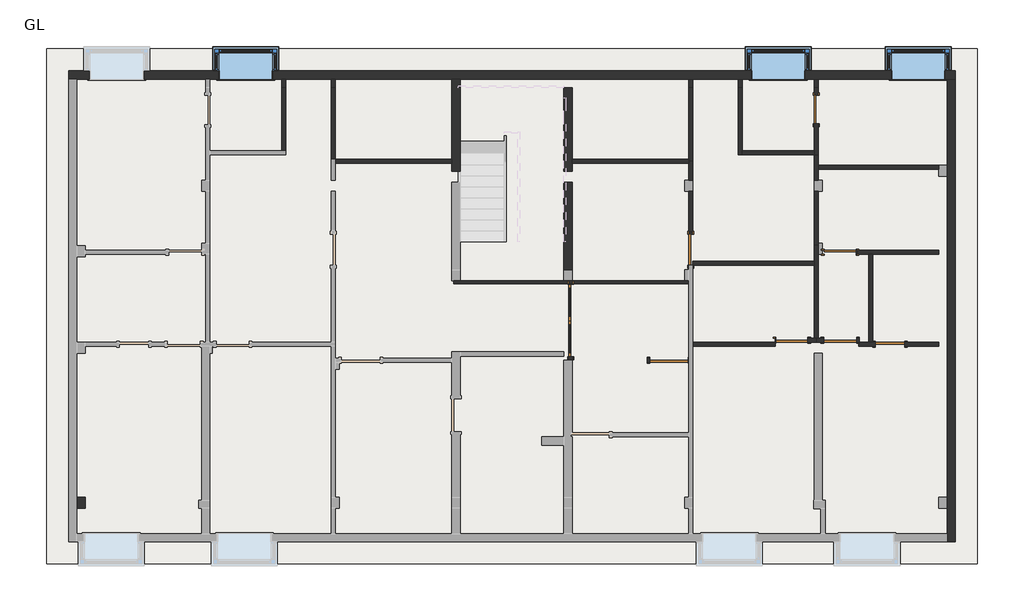
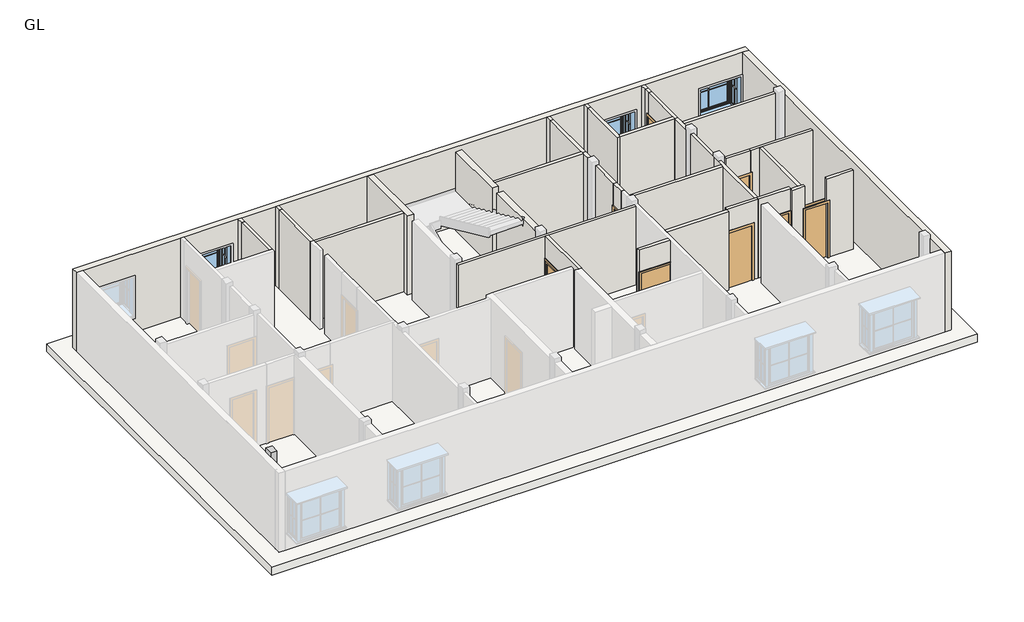
# One storey, part 2 of 3: 38 walls, 8 doors, 3 windows, 1 column, 1 slab.
"""IFC4 building model written with IfcOpenShell, lengths in millimetres."""

from ifc_helpers import new_model, si_unit, frame, origin, place, context, project, spatial, polyline, outline, extrude, faceted_brep, transform, mapped, element, save
from components import door_04ab2522, m_door_single_panel_05506f71, door_85b31ab1, door_1991e9a2, door_a431d384, door_82def9da, m_door_single_panel_3_x7_f8176753, window_19bbd869

model = new_model("IFC4")

# Units and contexts
model_context = context("Model", 3, world=origin())
ifc_project = project(units=[si_unit("LENGTHUNIT", "METRE", prefix="MILLI")], contexts=[model_context])

# Site, building, storey
site = spatial("IfcSite", under=ifc_project)
building = spatial("IfcBuilding", under=site)
storey = spatial("IfcBuildingStorey", under=building, Name="GL", Elevation=3200.4)

# Column
placement = place(None, origin())
element("IfcColumn", 1, ObjectType="Rectangular Column : 1'X 9\"", at=placement, inside=storey, context=model_context, shape_type="SweptSolid", body=[
    extrude(outline(polyline([(-12224.6987957, -3709.2932671), (-12224.6987957, -4014.0932671), (-12453.2987957, -4014.0932671), (-12453.2987957, -3709.2932671), (-12224.6987957, -3709.2932671)])), frame((0.0, 0.0, 3200.4), z_axis=(0.0, 0.0, 1.0), x_axis=(1.0, 0.0, 0.0)), (0.0, 0.0, 1.0), 3200.4),
])

# Doors
door_shape = door_04ab2522(model_context)
element("IfcDoor", 2, ObjectType="M_Door-Double-Glass : 6'7\"X7'", at=placement, inside=storey, context=model_context, shape_type="MappedRepresentation", body=[
    mapped(door_shape, transform((1217.5394962, 1183.3817656, 3200.4), x_axis=(0.0, 1.0, 0.0), y_axis=(-1.0, 0.0, 0.0), z_axis=(0.0, 0.0, 1.0))),
])
m_door_single_panel_shape = m_door_single_panel_05506f71(model_context)
element("IfcDoor", 3, ObjectType="M_Door-Single-Panel", at=placement, inside=storey, context=model_context, shape_type="MappedRepresentation", body=[
    mapped(m_door_single_panel_shape, transform((3933.4813133, 90.9578621, 3200.4), x_axis=(1.0, 0.0, 0.0), y_axis=(0.0, 1.0, 0.0), z_axis=(0.0, 0.0, 1.0))),
])
door_2_shape = door_85b31ab1(model_context)
element("IfcDoor", 4, ObjectType="M_Door-Single-Panel : 2'10\"X7' 2", at=placement, inside=storey, context=model_context, shape_type="MappedRepresentation", body=[
    mapped(door_2_shape, transform((4532.9512082, 3142.9626891, 3200.4), x_axis=(0.0, -1.0, 0.0), y_axis=(1.0, 0.0, 0.0), z_axis=(0.0, 0.0, 1.0))),
])
door_3_shape = door_1991e9a2(model_context)
element("IfcDoor", 5, ObjectType="M_Door-Single-Panel : 2'11\"X7' 3", at=placement, inside=storey, context=model_context, shape_type="MappedRepresentation", body=[
    mapped(door_3_shape, transform((7330.1405552, 640.4567334, 3200.4), x_axis=(1.0, 0.0, 0.0), y_axis=(0.0, 1.0, 0.0), z_axis=(0.0, 0.0, 1.0))),
])
element("IfcDoor", 6, ObjectType="M_Door-Single-Panel : 2'11\"X7' 3", at=placement, inside=storey, context=model_context, shape_type="MappedRepresentation", body=[
    mapped(door_3_shape, transform((8664.274939, 3078.8567332, 3200.4), x_axis=(-1.0, 0.0, 0.0), y_axis=(0.0, -1.0, 0.0), z_axis=(0.0, 0.0, 1.0))),
])
door_4_shape = door_a431d384(model_context)
element("IfcDoor", 7, ObjectType="M_Door-Single-Panel : 2'7\"X7' 2", at=placement, inside=storey, context=model_context, shape_type="MappedRepresentation", body=[
    mapped(door_4_shape, transform((8000.0512079, 7021.3751452, 3200.4), x_axis=(0.0, 1.0, 0.0), y_axis=(-1.0, 0.0, 0.0), z_axis=(0.0, 0.0, 1.0))),
])
door_5_shape = door_82def9da(model_context)
element("IfcDoor", 8, ObjectType="M_Door-Single-Panel : 2'8\"X7'", at=placement, inside=storey, context=model_context, shape_type="MappedRepresentation", body=[
    mapped(door_5_shape, transform((10046.0486694, 526.1567295, 3200.4), x_axis=(-1.0, 0.0, 0.0), y_axis=(0.0, -1.0, 0.0), z_axis=(0.0, 0.0, 1.0))),
])
m_door_single_panel_3_x7_shape = m_door_single_panel_3_x7_f8176753(model_context)
element("IfcDoor", 9, ObjectType="M_Door-Single-Panel : 3'X7'", at=placement, inside=storey, context=model_context, shape_type="MappedRepresentation", body=[
    mapped(m_door_single_panel_3_x7_shape, transform((8666.8012079, 640.4567334, 3200.4), x_axis=(-1.0, 0.0, 0.0), y_axis=(0.0, -1.0, 0.0), z_axis=(0.0, 0.0, 1.0))),
])

# Slab
element("IfcSlab", 10, ObjectType="Generic - 12\"", at=placement, inside=storey, context=model_context, shape_type="SweptSolid", body=[
    extrude(outline(polyline([(12464.1012075, 8698.6067329), (12464.1012075, -5550.7932662), (-13291.4987957, -5550.7932662), (-13291.4987957, 8698.6067329), (12464.1012075, 8698.6067329)])), frame((0.0, 0.0, 2895.6), z_axis=(0.0, 0.0, 1.0), x_axis=(1.0, 0.0, 0.0)), (0.0, 0.0, 1.0), 304.8),
])

# Walls
element("IfcWall", 11, ObjectType="3.5\"", at=placement, inside=storey, context=model_context, shape_type="Brep", body=[
    faceted_brep([(-2020.2487998, 2196.2067742, 3200.4), (1158.0082462, 2196.2067742, 3200.4), (1272.3082462, 2196.2067742, 3200.4), (4475.8012082, 2196.2067742, 3200.4), (4475.8012082, 2196.2067742, 6248.4), (1272.3082462, 2196.2067742, 6248.4), (1158.0082462, 2196.2067742, 6248.4), (-2020.2487998, 2196.2067742, 6248.4), (-2020.2487998, 2285.1067742, 3200.4), (-2020.2487998, 2285.1067742, 6248.4), (4475.8012082, 2285.1067742, 6248.4), (4475.8012082, 2285.1067742, 3200.4), (4361.5012082, 2285.1067742, 3200.4), (1253.2582462, 2285.1067742, 3200.4), (1024.6582462, 2285.1067742, 3200.4), (-1845.5417538, 2285.1067742, 3200.4)], [[[0, 1, 2, 3, 4, 5, 6, 7]], [[8, 9, 10, 11, 12, 13, 14, 15]], [[3, 2, 1, 0, 8, 15, 14, 13, 12, 11]], [[7, 6, 5, 4, 10, 9]], [[0, 7, 9, 8]], [[4, 3, 11, 10]]]),
])
element("IfcWall", 12, ObjectType="4.5\"", at=placement, inside=storey, context=model_context, shape_type="SweptSolid", body=[
    extrude(outline(polyline([(3132.0737955, 6248.4), (3628.3344162, 6248.4), (3628.3344162, 3200.4), (3574.7626891, 3200.4), (3574.7626891, 5334.0), (3132.0737955, 5334.0), (3132.0737955, 6248.4)])), frame((4475.8012082, 0.0, 0.0), z_axis=(1.0, 0.0, 0.0), x_axis=(0.0, 1.0, 0.0)), (0.0, 0.0, 1.0), 114.3),
])
element("IfcWall", 13, ObjectType="4.5\"", at=placement, inside=storey, context=model_context, shape_type="Brep", body=[
    faceted_brep([(8000.0512079, 583.3067334, 3200.4), (8000.0512079, 583.3067334, 6248.4), (6862.7668241, 583.3067334, 6248.4), (6862.7668241, 583.3067334, 3200.4), (6885.6405552, 583.3067334, 3200.4), (6885.6405552, 583.3067334, 5334.0), (7774.6405552, 583.3067334, 5334.0), (7774.6405552, 583.3067334, 3200.4), (8000.0512079, 697.6067334, 6248.4), (8000.0512079, 697.6067334, 3200.4), (7942.9012079, 697.6067334, 3200.4), (7774.6405552, 697.6067334, 3200.4), (7774.6405552, 697.6067334, 5334.0), (6885.6405552, 697.6067334, 5334.0), (6885.6405552, 697.6067334, 3200.4), (6862.7668241, 697.6067334, 3200.4), (6862.7668241, 697.6067334, 6248.4), (7942.9012079, 697.6067334, 6248.4)], [[[0, 1, 2, 3, 4, 5, 6, 7]], [[8, 9, 10, 11, 12, 13, 14, 15, 16, 17]], [[3, 15, 14, 4]], [[9, 0, 7, 11, 10]], [[1, 0, 9, 8]], [[2, 1, 8, 17, 16]], [[3, 2, 16, 15]], [[6, 12, 11, 7]], [[12, 6, 5, 13]], [[13, 5, 4, 14]]]),
])
element("IfcWall", 14, ObjectType="4.5\"", at=placement, inside=storey, context=model_context, shape_type="Brep", body=[
    faceted_brep([(9187.5012047, 583.3067334, 3200.4), (9187.5012047, 583.3067334, 6248.4), (8000.0512079, 583.3067334, 6248.4), (8000.0512079, 583.3067334, 3200.4), (8209.6012079, 583.3067334, 3200.4), (8209.6012079, 583.3067334, 5334.0), (9124.0012079, 583.3067334, 5334.0), (9124.0012079, 583.3067334, 3200.4), (9187.5012047, 697.6067334, 6248.4), (9187.5012047, 697.6067334, 3200.4), (9124.0012079, 697.6067334, 3200.4), (9124.0012079, 697.6067334, 5334.0), (8209.6012079, 697.6067334, 5334.0), (8209.6012079, 697.6067334, 3200.4), (8057.2012079, 697.6067334, 3200.4), (8000.0512079, 697.6067334, 3200.4), (8000.0512079, 697.6067334, 6248.4), (8057.2012079, 697.6067334, 6248.4)], [[[0, 1, 2, 3, 4, 5, 6, 7]], [[8, 9, 10, 11, 12, 13, 14, 15, 16, 17]], [[9, 0, 7, 10]], [[3, 15, 14, 13, 4]], [[1, 0, 9, 8]], [[2, 1, 8, 17, 16]], [[3, 2, 16, 15]], [[5, 12, 11, 6]], [[6, 11, 10, 7]], [[12, 5, 4, 13]]]),
])
element("IfcWall", 15, ObjectType="4.5\"", at=placement, inside=storey, context=model_context, shape_type="SweptSolid", body=[
    extrude(outline(polyline([(3200.4, 9131.6486701), (6248.4, 9131.6486701), (6248.4, 8245.174939), (5334.0, 8245.174939), (5334.0, 9108.774939), (3200.4, 9108.774939), (3200.4, 9131.6486701)])), frame((0.0, 3021.7067332, 0.0), z_axis=(0.0, 1.0, 0.0), x_axis=(0.0, 0.0, 1.0)), (0.0, 0.0, 1.0), 114.3),
])
element("IfcWall", 16, ObjectType="4.5\"", at=placement, inside=storey, context=model_context, shape_type="Brep", body=[
    faceted_brep([(7942.9012079, 5764.9067329, 6248.4), (7942.9012079, 5879.2067329, 6248.4), (7942.9012079, 7415.0751452, 6248.4), (7942.9012079, 7415.0751452, 5334.0), (7942.9012079, 6627.6751452, 5334.0), (7942.9012079, 6627.6751452, 3200.4), (7942.9012079, 5879.2067329, 3200.4), (7942.9012079, 5764.9067329, 3200.4), (8057.2012079, 7415.0751452, 6248.4), (8057.2012079, 5764.9067329, 6248.4), (8057.2012079, 5764.9067329, 3200.4), (8057.2012079, 6627.6751452, 3200.4), (8057.2012079, 6627.6751452, 5334.0), (8057.2012079, 7415.0751452, 5334.0)], [[[0, 1, 2, 3, 4, 5, 6, 7]], [[8, 9, 10, 11, 12, 13]], [[10, 7, 6, 5, 11]], [[2, 1, 0, 9, 8]], [[2, 8, 13, 3]], [[12, 4, 3, 13]], [[4, 12, 11, 5]], [[0, 7, 10, 9]]]),
])
element("IfcWall", 17, ObjectType="4.5\"", at=placement, inside=storey, context=model_context, shape_type="SweptSolid", body=[
    extrude(outline(polyline([(5334.0, 4466.8813133), (3200.4, 4466.8813133), (3200.4, 4475.8012082), (6248.4, 4475.8012082), (6248.4, 3334.0114184), (3200.4, 3334.0114184), (3200.4, 3400.0813133), (5334.0, 3400.0813133), (5334.0, 4466.8813133)])), frame((0.0, 33.8078621, 0.0), z_axis=(0.0, 1.0, 0.0), x_axis=(0.0, 0.0, 1.0)), (0.0, 0.0, 1.0), 114.3),
])
element("IfcWall", 18, ObjectType="4.5\"", at=placement, inside=storey, context=model_context, shape_type="Brep", body=[
    faceted_brep([(1158.0082462, 2196.2067742, 3200.4), (1158.0082462, 2186.6817656, 3200.4), (1158.0082462, 2186.6817656, 5334.0), (1158.0082462, 180.0817656, 5334.0), (1158.0082462, 180.0817656, 3200.4), (1158.0082462, 90.9578621, 3200.4), (1158.0082462, 90.9578621, 6248.4), (1158.0082462, 2196.2067742, 6248.4), (1272.3082462, 2186.6817656, 5334.0), (1272.3082462, 2186.6817656, 3200.4), (1272.3082462, 2196.2067742, 3200.4), (1272.3082462, 2196.2067742, 6248.4), (1272.3082462, 90.9578621, 6248.4), (1272.3082462, 90.9578621, 3200.4), (1272.3082462, 180.0817656, 3200.4), (1272.3082462, 180.0817656, 5334.0), (1250.0012085, 90.9578621, 3200.4), (1250.0012085, 90.9578621, 6248.4)], [[[0, 1, 2, 3, 4, 5, 6, 7]], [[8, 9, 10, 11, 12, 13, 14, 15]], [[14, 13, 16, 5, 4]], [[10, 9, 1, 0]], [[6, 5, 16, 13, 12, 17]], [[7, 6, 17, 12, 11]], [[2, 1, 9, 8]], [[3, 2, 8, 15]], [[4, 3, 15, 14]], [[0, 7, 11, 10]]]),
])
element("IfcWall", 19, ObjectType="4.5\"", at=placement, inside=storey, context=model_context, shape_type="Brep", body=[
    faceted_brep([(1250.0012085, 5536.3067329, 3200.4), (4475.8012082, 5536.3067329, 3200.4), (4475.8012082, 5536.3067329, 6248.4), (1250.0012085, 5536.3067329, 6248.4), (1250.0012085, 5650.6067329, 3200.4), (1250.0012085, 5650.6067329, 6248.4), (4475.8012082, 5650.6067329, 6248.4), (4475.8012082, 5650.6067329, 3200.4), (4475.8012082, 5593.4567329, 3200.4), (4475.8012082, 5593.4567329, 6248.4)], [[[0, 1, 2, 3]], [[4, 5, 6, 7]], [[1, 0, 4, 7, 8]], [[3, 2, 9, 6, 5]], [[2, 1, 8, 7, 6, 9]], [[0, 3, 5, 4]]]),
])
element("IfcWall", 20, ObjectType="4.5\"", at=placement, inside=storey, context=model_context, shape_type="Brep", body=[
    faceted_brep([(7942.9012079, 7631.8067329, 3200.4), (7942.9012079, 7415.0751452, 3200.4), (7942.9012079, 7415.0751452, 5334.0), (7942.9012079, 7415.0751452, 6248.4), (7942.9012079, 7631.8067329, 6248.4), (8057.2012079, 7631.8067329, 3200.4), (8057.2012079, 7631.8067329, 6248.4), (8057.2012079, 7415.0751452, 6248.4), (8057.2012079, 7415.0751452, 5334.0), (8057.2012079, 7415.0751452, 3200.4)], [[[0, 1, 2, 3, 4]], [[5, 6, 7, 8, 9]], [[1, 0, 5, 9]], [[3, 2, 1, 9, 8, 7]], [[4, 3, 7, 6]], [[0, 4, 6, 5]]]),
])
element("IfcWall", 21, ObjectType="4.5\"", at=placement, inside=storey, context=model_context, shape_type="Brep", body=[
    faceted_brep([(8057.2012047, 3270.1432417, 3200.4), (8057.2012047, 3326.5067332, 3200.4), (8057.2012047, 4760.6824989, 3200.4), (8057.2012047, 4760.6824989, 6248.4), (8057.2012047, 3326.5067332, 6248.4), (8057.2012047, 3270.1432417, 6248.4), (7942.9012047, 3270.1432417, 3200.4), (7942.9012047, 3270.1432417, 6248.4), (7942.9012047, 3326.5067332, 6248.4), (7942.9012047, 4760.6824989, 6248.4), (7942.9012047, 4760.6824989, 3200.4), (7943.9040565, 4760.6824989, 3200.4)], [[[0, 1, 2, 3, 4, 5]], [[6, 7, 8, 9, 10]], [[2, 1, 0, 6, 10, 11]], [[3, 2, 11, 10, 9]], [[5, 4, 3, 9, 8, 7]], [[0, 5, 7, 6]]]),
])
element("IfcWall", 22, ObjectType="4.5\"", at=placement, inside=storey, context=model_context, shape_type="Brep", body=[
    faceted_brep([(7942.9012079, 3270.1432417, 3200.4), (7942.9012079, 2825.4626891, 3200.4), (7942.9012079, 2711.1626891, 3200.4), (7942.9012079, 697.6067334, 3200.4), (7942.9012079, 697.6067334, 6248.4), (7942.9012079, 2711.1626891, 6248.4), (7942.9012079, 2825.4626891, 6248.4), (7942.9012079, 3270.1432417, 6248.4), (8057.2012079, 3270.1432417, 3200.4), (8057.2012079, 3270.1432417, 6248.4), (8057.2012079, 3021.7067332, 6248.4), (8057.2012079, 697.6067334, 6248.4), (8057.2012079, 697.6067334, 3200.4), (8057.2012079, 3021.7067332, 3200.4), (8000.0512079, 697.6067334, 3200.4), (8000.0512079, 697.6067334, 6248.4)], [[[0, 1, 2, 3, 4, 5, 6, 7]], [[8, 9, 10, 11, 12, 13]], [[3, 2, 1, 0, 8, 13, 12, 14]], [[7, 6, 5, 4, 15, 11, 10, 9]], [[0, 7, 9, 8]], [[4, 3, 14, 12, 11, 15]]]),
])
element("IfcWall", 23, ObjectType="4.5\"", at=placement, inside=storey, context=model_context, shape_type="Brep", body=[
    faceted_brep([(8058.2040565, 5065.4824989, 3200.4), (8058.2040565, 5364.8567329, 3200.4), (8058.2040565, 5479.1567329, 3200.4), (8058.2040565, 5763.9824989, 3200.4), (8058.2040565, 5763.9824989, 6248.4), (8058.2040565, 5479.1567329, 6248.4), (8058.2040565, 5364.8567329, 6248.4), (8058.2040565, 5065.4824989, 6248.4), (7943.9040565, 5065.4824989, 3200.4), (7943.9040565, 5065.4824989, 6248.4), (7943.9040565, 5763.9824989, 6248.4), (7943.9040565, 5763.9824989, 3200.4)], [[[0, 1, 2, 3, 4, 5, 6, 7]], [[8, 9, 10, 11]], [[3, 2, 1, 0, 8, 11]], [[4, 3, 11, 10]], [[7, 6, 5, 4, 10, 9]], [[0, 7, 9, 8]]]),
])
element("IfcWall", 24, ObjectType="4.5\"", at=placement, inside=storey, context=model_context, shape_type="SweptSolid", body=[
    extrude(outline(polyline([(-6674.7987994, 7860.4067329), (-6674.7987994, 7631.8067329), (-6789.0987994, 7631.8067329), (-6789.0987994, 7860.4067329), (-6674.7987994, 7860.4067329)])), frame((0.0, 0.0, 3200.4), z_axis=(0.0, 0.0, 1.0), x_axis=(1.0, 0.0, 0.0)), (0.0, 0.0, 1.0), 3048.0),
])
element("IfcWall", 25, ObjectType="4.5\"", at=placement, inside=storey, context=model_context, shape_type="SweptSolid", body=[
    extrude(outline(polyline([(-5303.1987995, 7860.4067329), (-5303.1987995, 7631.8067329), (-5417.4987995, 7631.8067329), (-5417.4987995, 7860.4067329), (-5303.1987995, 7860.4067329)])), frame((0.0, 0.0, 3200.4), z_axis=(0.0, 0.0, 1.0), x_axis=(1.0, 0.0, 0.0)), (0.0, 0.0, 1.0), 3048.0),
])
element("IfcWall", 26, ObjectType="4.5\"", at=placement, inside=storey, context=model_context, shape_type="SweptSolid", body=[
    extrude(outline(polyline([(4590.1012082, 7860.4067329), (4590.1012082, 7631.8067329), (4475.8012082, 7631.8067329), (4475.8012082, 7860.4067329), (4590.1012082, 7860.4067329)])), frame((0.0, 0.0, 3200.4), z_axis=(0.0, 0.0, 1.0), x_axis=(1.0, 0.0, 0.0)), (0.0, 0.0, 1.0), 3048.0),
])
element("IfcWall", 27, ObjectType="4.5\"", at=placement, inside=storey, context=model_context, shape_type="SweptSolid", body=[
    extrude(outline(polyline([(5961.701208, 7860.4067329), (5961.701208, 7631.8067329), (5847.401208, 7631.8067329), (5847.401208, 7860.4067329), (5961.701208, 7860.4067329)])), frame((0.0, 0.0, 3200.4), z_axis=(0.0, 0.0, 1.0), x_axis=(1.0, 0.0, 0.0)), (0.0, 0.0, 1.0), 3048.0),
])
element("IfcWall", 28, ObjectType="4.5\"", at=placement, inside=storey, context=model_context, shape_type="SweptSolid", body=[
    extrude(outline(polyline([(8057.2012079, 7860.4067329), (8057.2012079, 7631.8067329), (7942.9012079, 7631.8067329), (7942.9012079, 7860.4067329), (8057.2012079, 7860.4067329)])), frame((0.0, 0.0, 3200.4), z_axis=(0.0, 0.0, 1.0), x_axis=(1.0, 0.0, 0.0)), (0.0, 0.0, 1.0), 3048.0),
])
element("IfcWall", 29, ObjectType="4.5\"", at=placement, inside=storey, context=model_context, shape_type="SweptSolid", body=[
    extrude(outline(polyline([(8058.2040565, 5479.1567329), (11397.3012075, 5479.1567329), (11397.3012075, 5364.8567329), (8058.2040565, 5364.8567329), (8058.2040565, 5479.1567329)])), frame((0.0, 0.0, 3200.4), z_axis=(0.0, 0.0, 1.0), x_axis=(1.0, 0.0, 0.0)), (0.0, 0.0, 1.0), 3048.0),
])
element("IfcWall", 30, ObjectType="4.5\"", at=placement, inside=storey, context=model_context, shape_type="SweptSolid", body=[
    extrude(outline(polyline([(7942.9012079, 2711.1626891), (4590.1012082, 2711.1626891), (4590.1012082, 2825.4626891), (7942.9012079, 2825.4626891), (7942.9012079, 2711.1626891)])), frame((0.0, 0.0, 3200.4), z_axis=(0.0, 0.0, 1.0), x_axis=(1.0, 0.0, 0.0)), (0.0, 0.0, 1.0), 3048.0),
])
element("IfcWall", 31, ObjectType="4.5\" 2", at=placement, inside=storey, context=model_context, shape_type="SweptSolid", body=[
    extrude(outline(polyline([(-6674.7987994, 7631.8067329), (-6674.7987994, 5879.2067329), (-6789.0987994, 5879.2067329), (-6789.0987994, 7631.8067329), (-6674.7987994, 7631.8067329)])), frame((0.0, 0.0, 3200.4), z_axis=(0.0, 0.0, 1.0), x_axis=(1.0, 0.0, 0.0)), (0.0, 0.0, 1.0), 3048.0),
])
element("IfcWall", 32, ObjectType="4.5\" 2", at=placement, inside=storey, context=model_context, shape_type="SweptSolid", body=[
    extrude(outline(polyline([(-2077.3987998, 5536.3067329), (-5303.1987995, 5536.3067329), (-5303.1987995, 5650.6067329), (-2077.3987998, 5650.6067329), (-2077.3987998, 5536.3067329)])), frame((0.0, 0.0, 3200.4), z_axis=(0.0, 0.0, 1.0), x_axis=(1.0, 0.0, 0.0)), (0.0, 0.0, 1.0), 3048.0),
])
element("IfcWall", 33, ObjectType="4.5\" 2", at=placement, inside=storey, context=model_context, shape_type="SweptSolid", body=[
    extrude(outline(polyline([(-5417.4987995, 5650.6067329), (-5417.4987995, 7631.8067329), (-5303.1987995, 7631.8067329), (-5303.1987995, 5650.6067329), (-5417.4987995, 5650.6067329)])), frame((0.0, 0.0, 3200.4), z_axis=(0.0, 0.0, 1.0), x_axis=(1.0, 0.0, 0.0)), (0.0, 0.0, 1.0), 3048.0),
])
element("IfcWall", 34, ObjectType="4.5\" 2", at=placement, inside=storey, context=model_context, shape_type="Brep", body=[
    faceted_brep([(4475.8012082, 5593.4567329, 3200.4), (4475.8012082, 5536.3067329, 3200.4), (4475.8012082, 5066.40678, 3200.4), (4475.8012082, 5066.40678, 6248.4), (4475.8012082, 5536.3067329, 6248.4), (4475.8012082, 5593.4567329, 6248.4), (4590.1012082, 5593.4567329, 3200.4), (4590.1012082, 5593.4567329, 6248.4), (4590.1012082, 5066.40678, 6248.4), (4590.1012082, 5066.40678, 3200.4)], [[[0, 1, 2, 3, 4, 5]], [[6, 7, 8, 9]], [[2, 1, 0, 6, 9]], [[3, 2, 9, 8]], [[5, 4, 3, 8, 7]], [[0, 5, 7, 6]]]),
])
element("IfcWall", 35, ObjectType="4.5\" 2", at=placement, inside=storey, context=model_context, shape_type="SweptSolid", body=[
    extrude(outline(polyline([(4475.8012082, 3628.3344162), (4475.8012082, 4761.606733), (4590.1012082, 4761.606733), (4590.1012082, 3628.3344162), (4475.8012082, 3628.3344162)])), frame((0.0, 0.0, 3200.4), z_axis=(0.0, 0.0, 1.0), x_axis=(1.0, 0.0, 0.0)), (0.0, 0.0, 1.0), 3048.0),
])
element("IfcWall", 36, ObjectType="4.5\" 2", at=placement, inside=storey, context=model_context, shape_type="SweptSolid", body=[
    extrude(outline(polyline([(6862.7668241, 469.0067334), (4590.1012082, 469.0067334), (4590.1012082, 583.3067334), (6862.7668241, 583.3067334), (6862.7668241, 469.0067334)])), frame((0.0, 0.0, 3200.4), z_axis=(0.0, 0.0, 1.0), x_axis=(1.0, 0.0, 0.0)), (0.0, 0.0, 1.0), 3048.0),
])
element("IfcWall", 37, ObjectType="4.5\" 2", at=placement, inside=storey, context=model_context, shape_type="Brep", body=[
    faceted_brep([(9182.4486694, 469.0067295, 3200.4), (9639.6486694, 469.0067295, 3200.4), (9639.6486694, 469.0067295, 6248.4), (9182.4486694, 469.0067295, 6248.4), (9182.4486694, 583.3067295, 3200.4), (9182.4486694, 583.3067295, 6248.4), (9451.1098918, 583.3067295, 6248.4), (9565.4098918, 583.3067295, 6248.4), (9639.6486694, 583.3067295, 6248.4), (9639.6486694, 583.3067295, 3200.4), (9565.4098918, 583.3067295, 3200.4), (9451.1098918, 583.3067295, 3200.4)], [[[0, 1, 2, 3]], [[4, 5, 6, 7, 8, 9, 10, 11]], [[1, 0, 4, 11, 10, 9]], [[2, 1, 9, 8]], [[3, 2, 8, 7, 6, 5]], [[0, 3, 5, 4]]]),
])
element("IfcWall", 38, ObjectType="4.5\" 2", at=placement, inside=storey, context=model_context, shape_type="SweptSolid", body=[
    extrude(outline(polyline([(3200.4, 11397.3012075), (6248.4, 11397.3012075), (6248.4, 10443.8236977), (5334.0, 10443.8236977), (5334.0, 10452.4486694), (3200.4, 10452.4486694), (3200.4, 11397.3012075)])), frame((0.0, 469.0067295, 0.0), z_axis=(0.0, 1.0, 0.0), x_axis=(0.0, 0.0, 1.0)), (0.0, 0.0, 1.0), 114.3),
])
element("IfcWall", 39, ObjectType="4.5\" 2", at=placement, inside=storey, context=model_context, shape_type="SweptSolid", body=[
    extrude(outline(polyline([(9565.4098918, 3021.7067332), (9565.4098918, 583.3067295), (9451.1098918, 583.3067295), (9451.1098918, 3021.7067332), (9565.4098918, 3021.7067332)])), frame((0.0, 0.0, 3200.4), z_axis=(0.0, 0.0, 1.0), x_axis=(1.0, 0.0, 0.0)), (0.0, 0.0, 1.0), 3048.0),
])
element("IfcWall", 40, ObjectType="4.5\" 2", at=placement, inside=storey, context=model_context, shape_type="Brep", body=[
    faceted_brep([(9131.6486701, 3021.7067332, 3200.4), (9451.1098918, 3021.7067332, 3200.4), (9565.4098918, 3021.7067332, 3200.4), (11397.3012075, 3021.7067332, 3200.4), (11397.3012075, 3021.7067332, 6248.4), (9565.4098918, 3021.7067332, 6248.4), (9451.1098918, 3021.7067332, 6248.4), (9131.6486701, 3021.7067332, 6248.4), (9131.6486701, 3136.0067332, 3200.4), (9131.6486701, 3136.0067332, 6248.4), (11397.3012075, 3136.0067332, 6248.4), (11397.3012075, 3136.0067332, 3200.4)], [[[0, 1, 2, 3, 4, 5, 6, 7]], [[8, 9, 10, 11]], [[3, 2, 1, 0, 8, 11]], [[4, 3, 11, 10]], [[7, 6, 5, 4, 10, 9]], [[0, 7, 9, 8]]]),
])
element("IfcWall", 41, ObjectType="4.5\" 2", at=placement, inside=storey, context=model_context, shape_type="Brep", body=[
    faceted_brep([(4590.1012082, 5593.4567329, 3200.4), (4590.1012082, 7631.8067329, 3200.4), (4590.1012082, 7631.8067329, 6248.4), (4590.1012082, 5593.4567329, 6248.4), (4475.8012082, 5593.4567329, 3200.4), (4475.8012082, 5593.4567329, 6248.4), (4475.8012082, 5650.6067329, 6248.4), (4475.8012082, 7631.8067329, 6248.4), (4475.8012082, 7631.8067329, 3200.4), (4475.8012082, 5650.6067329, 3200.4)], [[[0, 1, 2, 3]], [[4, 5, 6, 7, 8, 9]], [[1, 0, 4, 9, 8]], [[2, 1, 8, 7]], [[3, 2, 7, 6, 5]], [[0, 3, 5, 4]]]),
])
element("IfcWall", 42, ObjectType="4.5\" 2", at=placement, inside=storey, context=model_context, shape_type="Brep", body=[
    faceted_brep([(5847.401208, 7631.8067329, 3200.4), (5847.401208, 5764.9067329, 3200.4), (5847.401208, 5764.9067329, 6248.4), (5847.401208, 7631.8067329, 6248.4), (5961.701208, 7631.8067329, 3200.4), (5961.701208, 7631.8067329, 6248.4), (5961.701208, 5879.2067329, 6248.4), (5961.701208, 5764.9067329, 6248.4), (5961.701208, 5764.9067329, 3200.4), (5961.701208, 5879.2067329, 3200.4)], [[[0, 1, 2, 3]], [[4, 5, 6, 7, 8, 9]], [[1, 0, 4, 9, 8]], [[3, 2, 7, 6, 5]], [[0, 3, 5, 4]], [[2, 1, 8, 7]]]),
])
element("IfcWall", 43, ObjectType="4.5\" 2", at=placement, inside=storey, context=model_context, shape_type="SweptSolid", body=[
    extrude(outline(polyline([(7942.9012079, 5764.9067329), (5961.701208, 5764.9067329), (5961.701208, 5879.2067329), (7942.9012079, 5879.2067329), (7942.9012079, 5764.9067329)])), frame((0.0, 0.0, 3200.4), z_axis=(0.0, 0.0, 1.0), x_axis=(1.0, 0.0, 0.0)), (0.0, 0.0, 1.0), 3048.0),
])
element("IfcWall", 44, ObjectType="9\"", at=placement, inside=storey, context=model_context, shape_type="Brep", body=[
    faceted_brep([(-12681.8987957, 7860.4067329, 3200.4), (-12453.2987957, 7860.4067329, 3200.4), (-8884.5987992, 7860.4067329, 3200.4), (-8770.2987992, 7860.4067329, 3200.4), (-6789.0987994, 7860.4067329, 3200.4), (-6674.7987994, 7860.4067329, 3200.4), (-5417.4987995, 7860.4067329, 3200.4), (-5303.1987995, 7860.4067329, 3200.4), (-2074.1417538, 7860.4067329, 3200.4), (-1845.5417538, 7860.4067329, 3200.4), (4475.8012082, 7860.4067329, 3200.4), (4590.1012082, 7860.4067329, 3200.4), (5847.401208, 7860.4067329, 3200.4), (5961.701208, 7860.4067329, 3200.4), (7942.9012079, 7860.4067329, 3200.4), (8057.2012079, 7860.4067329, 3200.4), (11625.9012075, 7860.4067329, 3200.4), (11854.5012075, 7860.4067329, 3200.4), (11854.5012075, 7860.4067329, 6248.4), (11625.9012075, 7860.4067329, 6248.4), (8057.2012079, 7860.4067329, 6248.4), (7942.9012079, 7860.4067329, 6248.4), (5961.701208, 7860.4067329, 6248.4), (5847.401208, 7860.4067329, 6248.4), (4590.1012082, 7860.4067329, 6248.4), (4475.8012082, 7860.4067329, 6248.4), (-1845.5417538, 7860.4067329, 6248.4), (-2074.1417538, 7860.4067329, 6248.4), (-5303.1987995, 7860.4067329, 6248.4), (-5417.4987995, 7860.4067329, 6248.4), (-6674.7987994, 7860.4067329, 6248.4), (-6789.0987994, 7860.4067329, 6248.4), (-8770.2987992, 7860.4067329, 6248.4), (-8884.5987992, 7860.4067329, 6248.4), (-12453.2987957, 7860.4067329, 6248.4), (-12681.8987957, 7860.4067329, 6248.4), (-10598.3987957, 7860.4067329, 5351.2), (-10598.3987957, 7860.4067329, 3800.4), (-12098.3987957, 7860.4067329, 3800.4), (-12098.3987957, 7860.4067329, 5351.2), (-7029.6987993, 7860.4067329, 5351.2), (-7029.6987993, 7860.4067329, 3800.4), (-8529.6987993, 7860.4067329, 3800.4), (-8529.6987993, 7860.4067329, 5351.2), (7702.301208, 7860.4067329, 5351.2), (7702.301208, 7860.4067329, 3800.4), (6202.301208, 7860.4067329, 3800.4), (6202.301208, 7860.4067329, 5351.2), (11575.8012075, 7860.4067329, 5351.2), (11575.8012075, 7860.4067329, 3800.4), (10075.8012075, 7860.4067329, 3800.4), (10075.8012075, 7860.4067329, 5351.2), (-12681.8987957, 8089.0067329, 3200.4), (-12681.8987957, 8089.0067329, 6248.4), (11854.5012075, 8089.0067329, 6248.4), (11854.5012075, 8089.0067329, 3200.4), (-10598.3987957, 8089.0067329, 5351.2), (-12098.3987957, 8089.0067329, 5351.2), (-12098.3987957, 8089.0067329, 3800.4), (-10598.3987957, 8089.0067329, 3800.4), (-7029.6987993, 8089.0067329, 5351.2), (-8529.6987993, 8089.0067329, 5351.2), (-8529.6987993, 8089.0067329, 3800.4), (-7029.6987993, 8089.0067329, 3800.4), (7702.301208, 8089.0067329, 5351.2), (6202.301208, 8089.0067329, 5351.2), (6202.301208, 8089.0067329, 3800.4), (7702.301208, 8089.0067329, 3800.4), (11575.8012075, 8089.0067329, 5351.2), (10075.8012075, 8089.0067329, 5351.2), (10075.8012075, 8089.0067329, 3800.4), (11575.8012075, 8089.0067329, 3800.4)], [[[0, 1, 2, 3, 4, 5, 6, 7, 8, 9, 10, 11, 12, 13, 14, 15, 16, 17, 18, 19, 20, 21, 22, 23, 24, 25, 26, 27, 28, 29, 30, 31, 32, 33, 34, 35], [36, 37, 38, 39], [40, 41, 42, 43], [44, 45, 46, 47], [48, 49, 50, 51]], [[52, 53, 54, 55], [56, 57, 58, 59], [60, 61, 62, 63], [64, 65, 66, 67], [68, 69, 70, 71]], [[17, 16, 15, 14, 13, 12, 11, 10, 9, 8, 7, 6, 5, 4, 3, 2, 1, 0, 52, 55]], [[35, 34, 33, 32, 31, 30, 29, 28, 27, 26, 25, 24, 23, 22, 21, 20, 19, 18, 54, 53]], [[18, 17, 55, 54]], [[0, 35, 53, 52]], [[37, 36, 56, 59]], [[38, 37, 59, 58]], [[39, 38, 58, 57]], [[36, 39, 57, 56]], [[41, 40, 60, 63]], [[42, 41, 63, 62]], [[43, 42, 62, 61]], [[40, 43, 61, 60]], [[45, 44, 64, 67]], [[46, 45, 67, 66]], [[47, 46, 66, 65]], [[44, 47, 65, 64]], [[49, 48, 68, 71]], [[50, 49, 71, 70]], [[51, 50, 70, 69]], [[48, 51, 69, 68]]]),
])
element("IfcWall", 45, ObjectType="9\"", at=placement, inside=storey, context=model_context, shape_type="Brep", body=[
    faceted_brep([(11625.9012075, 7860.4067329, 3200.4), (11625.9012075, 5479.1567329, 3200.4), (11625.9012075, 5174.3567329, 3200.4), (11625.9012075, -3709.2932671, 3200.4), (11625.9012075, -4014.0932671, 3200.4), (11625.9012075, -4712.5932662, 3200.4), (11625.9012075, -4941.1932662, 3200.4), (11625.9012075, -4941.1932662, 6248.4), (11625.9012075, -4712.5932662, 6248.4), (11625.9012075, 7860.4067329, 6248.4), (11854.5012075, 7860.4067329, 3200.4), (11854.5012075, 7860.4067329, 6248.4), (11854.5012075, -4941.1932662, 6248.4), (11854.5012075, -4941.1932662, 3200.4)], [[[0, 1, 2, 3, 4, 5, 6, 7, 8, 9]], [[10, 11, 12, 13]], [[6, 5, 4, 3, 2, 1, 0, 10, 13]], [[9, 8, 7, 12, 11]], [[0, 9, 11, 10]], [[7, 6, 13, 12]]]),
])
element("IfcWall", 46, ObjectType="9\"", at=placement, inside=storey, context=model_context, shape_type="SweptSolid", body=[
    extrude(outline(polyline([(-2074.1417538, 5320.4067329), (-2074.1417538, 7860.4067329), (-1845.5417538, 7860.4067329), (-1845.5417538, 5320.4067329), (-2074.1417538, 5320.4067329)])), frame((0.0, 0.0, 3200.4), z_axis=(0.0, 0.0, 1.0), x_axis=(1.0, 0.0, 0.0)), (0.0, 0.0, 1.0), 3048.0),
])
element("IfcWall", 47, ObjectType="9\"", at=placement, inside=storey, context=model_context, shape_type="Brep", body=[
    faceted_brep([(1021.4012085, 7631.8067329, 3200.4), (1021.4012085, 5320.4067329, 3200.4), (1021.4012085, 5320.4067329, 6248.4), (1021.4012085, 7631.8067329, 6248.4), (1250.0012085, 7631.8067329, 3200.4), (1250.0012085, 7631.8067329, 6248.4), (1250.0012085, 5650.6067329, 6248.4), (1250.0012085, 5536.3067329, 6248.4), (1250.0012085, 5320.4067329, 6248.4), (1250.0012085, 5320.4067329, 3200.4), (1250.0012085, 5536.3067329, 3200.4), (1250.0012085, 5650.6067329, 3200.4)], [[[0, 1, 2, 3]], [[4, 5, 6, 7, 8, 9, 10, 11]], [[1, 0, 4, 11, 10, 9]], [[2, 1, 9, 8]], [[3, 2, 8, 7, 6, 5]], [[0, 3, 5, 4]]]),
])
element("IfcWall", 48, ObjectType="9\"", at=placement, inside=storey, context=model_context, shape_type="Brep", body=[
    faceted_brep([(1021.4012085, 5015.6067329, 3200.4), (1021.4012085, 2589.9067742, 3200.4), (1021.4012085, 2589.9067742, 6248.4), (1021.4012085, 5015.6067329, 6248.4), (1250.0012085, 5015.6067329, 3200.4), (1250.0012085, 5015.6067329, 6248.4), (1250.0012085, 2589.9067742, 6248.4), (1250.0012085, 2589.9067742, 3200.4), (1024.6582462, 2589.9067742, 3200.4)], [[[0, 1, 2, 3]], [[4, 5, 6, 7]], [[1, 0, 4, 7, 8]], [[2, 1, 8, 7, 6]], [[3, 2, 6, 5]], [[0, 3, 5, 4]]]),
])

# Windows
window_shape = window_19bbd869(model_context)
element("IfcWindow", 49, ObjectType="4'.8\"x3'.8\"", at=placement, inside=storey, context=model_context, shape_type="MappedRepresentation", body=[
    mapped(window_shape, transform((-7779.6987993, 7974.7067329, 3200.4), x_axis=(1.0, 0.0, 0.0), y_axis=(0.0, 1.0, 0.0), z_axis=(0.0, 0.0, 1.0))),
])
element("IfcWindow", 50, ObjectType="4'.8\"x3'.8\"", at=placement, inside=storey, context=model_context, shape_type="MappedRepresentation", body=[
    mapped(window_shape, transform((6952.301208, 7974.7067329, 3200.4), x_axis=(1.0, 0.0, 0.0), y_axis=(0.0, 1.0, 0.0), z_axis=(0.0, 0.0, 1.0))),
])
element("IfcWindow", 51, ObjectType="4'.8\"x3'.8\"", at=placement, inside=storey, context=model_context, shape_type="MappedRepresentation", body=[
    mapped(window_shape, transform((10825.8012075, 7974.7067329, 3200.4), x_axis=(1.0, 0.0, 0.0), y_axis=(0.0, 1.0, 0.0), z_axis=(0.0, 0.0, 1.0))),
])

save(model, "model.ifc")

# Revit data of these elements
# Type "Rectangular Column : 1'X 9\""
#   Assembly Code = "B1010200"
#   Depth = 1' - 0"
#   Offset Base = 0' - 0"
#   Offset Top = 0' - 0"
#   Width = 0' - 9"
#   Material = none
# Type "M_Door-Double-Glass : 6'7\"X7'"
#   Type Mark = "16"
#   Construction Type Id = "opn-d45"
#   Assembly Code = "C1020"
#   Analytic Construction = "Wood frame, double glass door "
#   W = 3' - 3 1/2"
#   Thickness = 0' - 1.9685"
#   Thermal Resistance (R) = 1.8150 (h·ft²·°F)/BTU
#   Swing Angle [instance default] = 90.00°
#   Heat Transfer Coefficient (U) = 0.5510 BTU/(h·ft²·°F)
#   Height = 7' - 0"
#   Bottom Rail = 0' - 3.93701"
#   Top Rail = 0' - 3.93701"
#   Stiles = 0' - 3.93701"
#   Trim Projection = 0' - 0.98425"
#   Trim Width = 0' - 3.14961"
#   Width = 6' - 7"
#   Define Thermal Properties by = 1
#   Glazing = Glass
#   Panel Material = Wood - Birch - Solid Stained Light Low Gloss
#   Trim Material = Paint - Sienna
#   Visual Light Transmittance = 0
#   Solar Heat Gain Coefficient = 0
#   Function = (empty or 0)
#   Wall Closure = (empty or 0)
# Type "M_Door-Single-Panel"
#   Type Mark = "14"
#   Construction Type Id = "DOOR"
#   Assembly Code = "C1020300"
#   Analytic Construction = "Wooden"
#   Thickness = 0' - 1.9685"
#   Thermal Resistance (R) = 2.5876 (h·ft²·°F)/BTU
#   Swing Angle [instance default] = 90.00°
#   Heat Transfer Coefficient (U) = 0.3865 BTU/(h·ft²·°F)
#   Height = 7' - 0"
#   Trim Projection Ext = 0' - 0.98425"
#   Trim Projection Int = 0' - 0.98425"
#   Trim Width = 0' - 3.14961"
#   Width = 3' - 6"
#   Define Thermal Properties by = 1
#   Panel Material = Wood - Birch - Solid Stained Light Low Gloss
#   Trim Material = Paint - Sienna
#   Visual Light Transmittance = 0
#   Solar Heat Gain Coefficient = 0
#   Function = (empty or 0)
#   Wall Closure = (empty or 0)
# Type "M_Door-Single-Panel : 2'10\"X7' 2"
#   Type Mark = "10"
#   Construction Type Id = "DOOR"
#   Assembly Code = "C1020300"
#   Analytic Construction = "Wooden"
#   Thickness = 0' - 1.9685"
#   Thermal Resistance (R) = 2.5876 (h·ft²·°F)/BTU
#   Swing Angle [instance default] = 90.00°
#   Heat Transfer Coefficient (U) = 0.3865 BTU/(h·ft²·°F)
#   Height = 7' - 0"
#   Trim Projection Ext = 0' - 0.98425"
#   Trim Projection Int = 0' - 0.98425"
#   Trim Width = 0' - 3.14961"
#   Width = 2' - 10"
#   Define Thermal Properties by = 1
#   Panel Material = Wood - Birch - Solid Stained Light Low Gloss
#   Trim Material = Paint - Sienna
#   Visual Light Transmittance = 0
#   Solar Heat Gain Coefficient = 0
#   Function = (empty or 0)
#   Wall Closure = (empty or 0)
# Type "M_Door-Single-Panel : 2'11\"X7' 3"
#   Type Mark = "12"
#   Construction Type Id = "DOOR"
#   Assembly Code = "C1020300"
#   Analytic Construction = "Wooden"
#   Thickness = 0' - 1.9685"
#   Thermal Resistance (R) = 2.5876 (h·ft²·°F)/BTU
#   Swing Angle [instance default] = 90.00°
#   Heat Transfer Coefficient (U) = 0.3865 BTU/(h·ft²·°F)
#   Height = 7' - 0"
#   Trim Projection Ext = 0' - 0.98425"
#   Trim Projection Int = 0' - 0.98425"
#   Trim Width = 0' - 3.14961"
#   Width = 2' - 11"
#   Define Thermal Properties by = 1
#   Panel Material = Wood - Birch - Solid Stained Light Low Gloss
#   Trim Material = Paint - Sienna
#   Visual Light Transmittance = 0
#   Solar Heat Gain Coefficient = 0
#   Function = (empty or 0)
#   Wall Closure = (empty or 0)
# Type "M_Door-Single-Panel : 2'7\"X7' 2"
#   Type Mark = "13"
#   Construction Type Id = "DOOR"
#   Assembly Code = "C1020300"
#   Analytic Construction = "Wooden"
#   Thickness = 0' - 1.9685"
#   Thermal Resistance (R) = 2.5876 (h·ft²·°F)/BTU
#   Swing Angle [instance default] = 90.00°
#   Heat Transfer Coefficient (U) = 0.3865 BTU/(h·ft²·°F)
#   Height = 7' - 0"
#   Trim Projection Ext = 0' - 0.98425"
#   Trim Projection Int = 0' - 0.98425"
#   Trim Width = 0' - 3.14961"
#   Width = 2' - 7"
#   Define Thermal Properties by = 1
#   Panel Material = Wood - Birch - Solid Stained Light Low Gloss
#   Trim Material = Paint - Sienna
#   Visual Light Transmittance = 0
#   Solar Heat Gain Coefficient = 0
#   Function = (empty or 0)
#   Wall Closure = (empty or 0)
# Type "M_Door-Single-Panel : 2'8\"X7'"
#   Type Mark = "9"
#   Construction Type Id = "DOOR"
#   Assembly Code = "C1020300"
#   Analytic Construction = "Wooden"
#   Thickness = 0' - 1.9685"
#   Thermal Resistance (R) = 2.5876 (h·ft²·°F)/BTU
#   Swing Angle [instance default] = 90.00°
#   Heat Transfer Coefficient (U) = 0.3865 BTU/(h·ft²·°F)
#   Height = 7' - 0"
#   Trim Projection Ext = 0' - 0.98425"
#   Trim Projection Int = 0' - 0.98425"
#   Trim Width = 0' - 3.14961"
#   Width = 2' - 8"
#   Define Thermal Properties by = 1
#   Panel Material = Wood - Birch - Solid Stained Light Low Gloss
#   Trim Material = Paint - Sienna
#   Visual Light Transmittance = 0
#   Solar Heat Gain Coefficient = 0
#   Function = (empty or 0)
#   Wall Closure = (empty or 0)
# Type "M_Door-Single-Panel : 3'X7'"
#   Type Mark = "11"
#   Construction Type Id = "DOOR"
#   Assembly Code = "C1020300"
#   Analytic Construction = "Wooden"
#   Thickness = 0' - 1.9685"
#   Thermal Resistance (R) = 2.5876 (h·ft²·°F)/BTU
#   Swing Angle [instance default] = 90.00°
#   Heat Transfer Coefficient (U) = 0.3865 BTU/(h·ft²·°F)
#   Height = 7' - 0"
#   Trim Projection Ext = 0' - 0.98425"
#   Trim Projection Int = 0' - 0.98425"
#   Trim Width = 0' - 3.14961"
#   Width = 3' - 0"
#   Define Thermal Properties by = 1
#   Panel Material = Wood - Birch - Solid Stained Light Low Gloss
#   Trim Material = Paint - Sienna
#   Visual Light Transmittance = 0
#   Solar Heat Gain Coefficient = 0
#   Function = (empty or 0)
#   Wall Closure = (empty or 0)
# Type "Generic - 12\""
#   Assembly Code = "B1010"
#   Function = 0
#   Layers, outside or top first: 1' - 0" no material (function 1)
# Type "3.5\""
#   Assembly Code = "B2010"
#   Layers, outside or top first: 0' - 3 1/2" no material (function 1)
# Type "4.5\""
#   Assembly Code = "B2010"
#   Layers, outside or top first: 0' - 4 1/2" no material (function 1)
# Type "4.5\" 2"
#   Assembly Code = "B2010"
#   Layers, outside or top first: 0' - 4 1/2" no material (function 1)
# Type "9\""
#   Assembly Code = "B2010"
#   Layers, outside or top first: 0' - 9" no material (function 1)
# Type "4'.8\"x3'.8\""
#   Type Mark = "20"
#   Fire Rating = "0.5h"
#   Assembly Code = "B2020100"
#   Analytic Construction = "1/8 in Pilkington single glazing"
#   Width = 4' - 11.05512"
#   Wall Thickness [instance default] = 0' - 5.90551"
#   Visual Light Transmittance = 0.9
#   Trim Width = 5' - 7.05512"
#   Trim Height = 4' - 11.05512"
#   Thermal Resistance (R) = 1.5394 (h·ft²·°F)/BTU
#   Solar Heat Gain Coefficient = 0.86
#   Rough Width = 4' - 11.64567"
#   Rough Height = 4' - 11.64567"
#   Height 1 = 5' - 1.05512"
#   Height = 4' - 11.05512"
#   Heat Transfer Coefficient (U) = 0.6496 BTU/(h·ft²·°F)
#   Depth = 1' - 11.62205"
#   Default Sill Height = 1' - 11.62205"
#   Side Muntin Visibility = yes
#   Center Muntin Visibility = yes
#   Interior Trim Visibility [instance default] = yes
#   Exterior Trim Visibility [instance default] = yes
#   Side Muntin Pattern = M_Muntin Pattern_2x2 : M_Muntin Pattern_2x2
#   Center Muntin Pattern = M_Muntin Pattern_2x2 : M_Muntin Pattern_2x2
#   Interior Trim Material = Wood - Stained
#   Exterior Trim Material = Clad - White
#   Exterior Trim = element 422966
#   Interior Trim = M_Trim-Window-Interior-Flat : Picture Frame
#   Interior Frame Material = Wood - Stained
#   Glass Panel Material = Glass
#   Exterior Frame Material = Clad - White
#   Wall Closure = (empty or 0)
# Element 1 (IfcColumn, "Rectangular Column : 1'X 9\"")
#   Phase Created = New Construction
#   Materials on its faces: "Default Wall"
# Element 2 (IfcDoor, "M_Door-Double-Glass : 6'7\"X7'")
#   Swing Angle = 90.00°
#   Phase Created = New Construction
#   Materials on its faces: "Wood - Birch - Solid Stained Light Low Gloss", "Paint - Sienna", "Glass"
# Element 3 (IfcDoor, "M_Door-Single-Panel")
#   Swing Angle = 90.00°
#   Phase Created = New Construction
#   Materials on its faces: "Paint - Sienna", "Wood - Birch - Solid Stained Light Low Gloss"
# Element 4 (IfcDoor, "M_Door-Single-Panel : 2'10\"X7' 2")
#   Swing Angle = 90.00°
#   Phase Created = New Construction
#   Materials on its faces: "Paint - Sienna", "Wood - Birch - Solid Stained Light Low Gloss"
# Elements 5, 6 (IfcDoor, "M_Door-Single-Panel : 2'11\"X7' 3")
#   Swing Angle = 90.00°
#   Phase Created = New Construction
#   Materials on its faces: "Paint - Sienna", "Wood - Birch - Solid Stained Light Low Gloss"
# Element 7 (IfcDoor, "M_Door-Single-Panel : 2'7\"X7' 2")
#   Swing Angle = 90.00°
#   Phase Created = New Construction
#   Materials on its faces: "Paint - Sienna", "Wood - Birch - Solid Stained Light Low Gloss"
# Element 8 (IfcDoor, "M_Door-Single-Panel : 2'8\"X7'")
#   Swing Angle = 90.00°
#   Phase Created = New Construction
#   Materials on its faces: "Paint - Sienna", "Wood - Birch - Solid Stained Light Low Gloss"
# Element 9 (IfcDoor, "M_Door-Single-Panel : 3'X7'")
#   Swing Angle = 90.00°
#   Phase Created = New Construction
#   Materials on its faces: "Paint - Sienna", "Wood - Birch - Solid Stained Light Low Gloss"
# Element 10 (IfcSlab, "Generic - 12\"")
#   Height Offset From Level = 0' - 0"
#   Phase Created = New Construction
#   Materials on its faces: "Default Floor"
# Element 11 (IfcWall, "3.5\"")
#   Top Offset = -0' - 6"
#   Base Offset = 0' - 0"
#   wall height = 10' - 0"
#   Phase Created = New Construction
#   Base Constraint = GL
#   Materials on its faces: "Default Wall"
# Elements 12, 13, 14, 15, 16, 17, 18, 19, 20, 21, 22, 23, 24, 25, 26, 27, 28, 29, 30 (IfcWall, "4.5\"")
#   Top Offset = -0' - 6"
#   Base Offset = 0' - 0"
#   wall height = 10' - 0"
#   Phase Created = New Construction
#   Base Constraint = GL
#   Materials on its faces: "Default Wall"
# Elements 31, 32, 33, 34, 35, 36, 37, 38, 39, 40, 41, 42, 43 (IfcWall, "4.5\" 2")
#   Top Offset = -0' - 6"
#   Base Offset = 0' - 0"
#   wall height = 10' - 0"
#   Phase Created = New Construction
#   Base Constraint = GL
#   Materials on its faces: "Default Wall"
# Elements 44, 45, 46, 47, 48 (IfcWall, "9\"")
#   Top Offset = -0' - 6"
#   Base Offset = 0' - 0"
#   wall height = 10' - 0"
#   Phase Created = New Construction
#   Base Constraint = GL
#   Materials on its faces: "Default Wall"
# Element 49 (IfcWindow, "4'.8\"x3'.8\"")
#   Mark = "272"
#   Interior Trim Visibility = yes
#   Exterior Trim Visibility = yes
#   Phase Created = New Construction
#   Materials on its faces: "Clad - White", "Wood - Stained", "Glass"
# Element 50 (IfcWindow, "4'.8\"x3'.8\"")
#   Mark = "273"
#   Interior Trim Visibility = yes
#   Exterior Trim Visibility = yes
#   Phase Created = New Construction
#   Materials on its faces: "Clad - White", "Wood - Stained", "Glass"
# Element 51 (IfcWindow, "4'.8\"x3'.8\"")
#   Mark = "274"
#   Interior Trim Visibility = yes
#   Exterior Trim Visibility = yes
#   Phase Created = New Construction
#   Materials on its faces: "Clad - White", "Wood - Stained", "Glass"
# Materials
#   "Glass": class "Glass", colour RGB 0 128 192, transparency 0.75, Description = "Soda Lime Glass", Cost = 0
#   "Wood - Birch - Solid Stained Light Low Gloss": class "Wood", colour RGB 210 159 95, transparency 0, Cost = 0
#   "Paint - Sienna": colour RGB 118 70 51, transparency 0, Cost = 0
#   "Wood - Stained": class "Wood", colour RGB 224 178 126, transparency 0, Cost = 0
#   "Clad - White": class "Wood", colour RGB 242 242 238, transparency 0, Cost = 0
#   "Default Wall": colour RGB 128 128 128, transparency 0, Cost = 0
#   "Default Floor": colour RGB 128 128 128, transparency 0, Cost = 0
